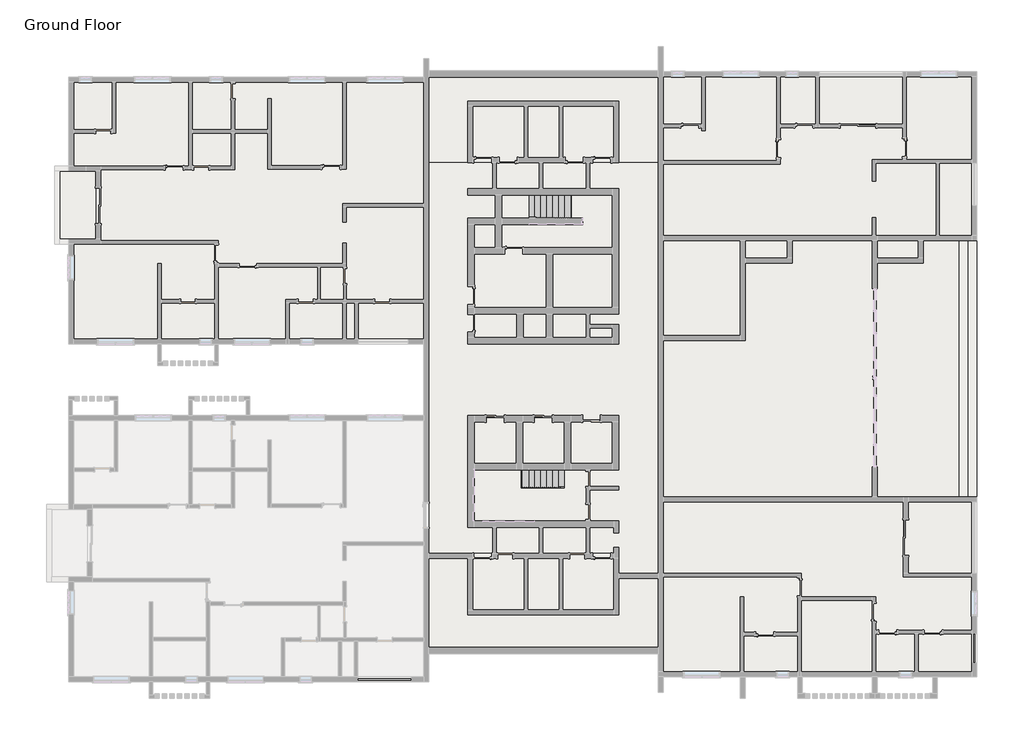
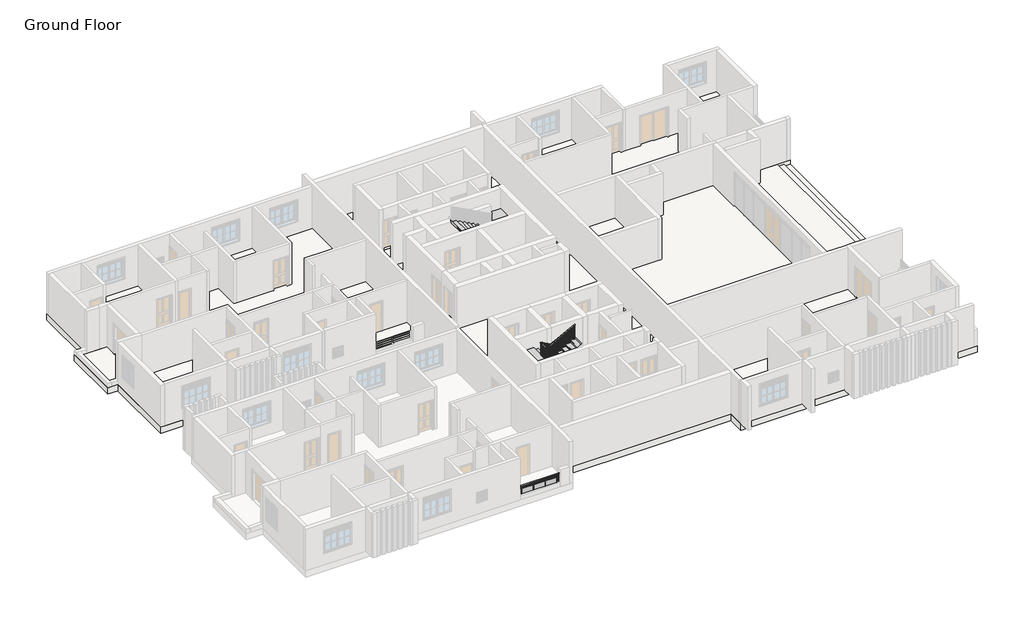
# One storey, part 6 of 9: 12 slabs, 3 railings, 2 stair flights.
"""IFC4 building model written with IfcOpenShell, lengths in millimetres."""

from ifc_helpers import new_model, si_unit, point, frame, frame_2d, origin, origin_with_axes, place, context, project, spatial, polyline, circle_curve, ellipse_curve, trimmed, segment, composite_curve, outline, extrude, faceted_brep, transform, mapped, element, save
from ifc_brep_helpers import plane_surface, extruded_surface, advanced_brep
from components import stair_flight_6b31ae14, stair_flight_54cbe99c

model = new_model("IFC4")

# Units and contexts
model_context = context("Model", 3, world=origin())
ifc_project = project(units=[si_unit("LENGTHUNIT", "METRE", prefix="MILLI")], contexts=[model_context])

# Site, building, storey
site = spatial("IfcSite", under=ifc_project)
building = spatial("IfcBuilding", under=site)
storey = spatial("IfcBuildingStorey", under=building, Name="Ground Floor", Elevation=0.0)

# Railings
placement = place(None, origin())
element("IfcRailing", 1, ObjectType="Glass Panel - Bottom Fill", at=placement, inside=storey, context=model_context, shape_type="SolidModel", body=[
    advanced_brep(
    [(403.2546318, -1832.865108, 914.4), (403.2546318, -1909.065108, 914.4), (3146.4546318, -1832.865108, 914.4), (3146.4546318, -1909.065108, 914.4)],
    [
        (0, 1, ellipse_curve(frame((403.2546318, -1870.965108, 914.4), z_axis=(-1.0, 0.0, 0.0), x_axis=(0.0, -1.0, 0.0)), 38.1, 28.575)),
        (1, 0, ellipse_curve(frame((403.2546318, -1870.965108, 914.4), z_axis=(-1.0, 0.0, 0.0), x_axis=(0.0, -1.0, 0.0)), 38.1, 28.575)),
        (2, 3, ellipse_curve(frame((3146.4546318, -1870.965108, 914.4), z_axis=(1.0, 0.0, 0.0), x_axis=(0.0, -1.0, 0.0)), 38.1, 28.575)),
        (3, 2, ellipse_curve(frame((3146.4546318, -1870.965108, 914.4), z_axis=(1.0, 0.0, 0.0), x_axis=(0.0, -1.0, 0.0)), 38.1, 28.575)),
        (0, 2),
        (3, 1),
    ],
    [
        plane_surface(frame((403.2546318, -1870.965108, 914.4), z_axis=(-1.0, 0.0, 0.0), x_axis=(0.0, 1.0, 0.0))),
        plane_surface(frame((3146.4546318, -1870.965108, 914.4), z_axis=(1.0, 0.0, 0.0), x_axis=(0.0, 1.0, 0.0))),
        extruded_surface(trimmed(ellipse_curve(frame((3146.4546318, -1870.965108, 914.4), z_axis=(-1.0, 0.0, 0.0), x_axis=(0.0, -1.0, 0.0)), 38.1, 28.575), [point((3146.4546318, -1832.865108, 914.4))], [point((3146.4546318, -1909.065108, 914.4))], True, "CARTESIAN"), (-2743.2, 0.0, 0.0), 2743.2),
        extruded_surface(trimmed(ellipse_curve(frame((3146.4546318, -1870.965108, 914.4), z_axis=(-1.0, 0.0, 0.0), x_axis=(0.0, -1.0, 0.0)), 38.1, 28.575), [point((3146.4546318, -1909.065108, 914.4))], [point((3146.4546318, -1832.865108, 914.4))], True, "CARTESIAN"), (-2743.2, 0.0, 0.0), 2743.2),
    ],
    [
        (0, [[1, 2]]),
        (1, [[3, 4]]),
        (2, [[-1, 5, -4, 6]]),
        (3, [[-2, -6, -3, -5]]),
    ],
),
    extrude(outline(polyline([(403.2546318, -1883.665108), (403.2546318, -1858.265108), (3146.4546318, -1858.265108), (3146.4546318, -1883.665108), (403.2546318, -1883.665108)])), frame((0.0, 0.0, 800.1), z_axis=(0.0, 0.0, 1.0), x_axis=(1.0, 0.0, 0.0)), (0.0, 0.0, 1.0), 25.4),
    extrude(outline(polyline([(403.2546318, -1883.665108), (403.2546318, -1858.265108), (3146.4546318, -1858.265108), (3146.4546318, -1883.665108), (403.2546318, -1883.665108)])), frame((0.0, 0.0, 698.5), z_axis=(0.0, 0.0, 1.0), x_axis=(1.0, 0.0, 0.0)), (0.0, 0.0, 1.0), 25.4),
    extrude(outline(polyline([(2987.7046318, -1896.365108), (2987.7046318, -1845.565108), (3000.4046318, -1845.565108), (3000.4046318, -1896.365108), (2987.7046318, -1896.365108)])), origin_with_axes(), (0.0, 0.0, 1.0), 885.825),
    extrude(outline(polyline([(2181.2546318, -1864.429951), (2994.0546318, -1864.429951), (2994.0546318, -1870.779951), (2181.2546318, -1870.779951), (2181.2546318, -1864.429951)])), frame((0.0, 0.0, 101.6), z_axis=(0.0, 0.0, 1.0), x_axis=(1.0, 0.0, 0.0)), (0.0, 0.0, 1.0), 596.9),
    extrude(outline(polyline([(2174.9046318, -1896.365108), (2174.9046318, -1845.565108), (2187.6046318, -1845.565108), (2187.6046318, -1896.365108), (2174.9046318, -1896.365108)])), origin_with_axes(), (0.0, 0.0, 1.0), 885.825),
    extrude(outline(polyline([(1368.4546318, -1864.429951), (2181.2546318, -1864.429951), (2181.2546318, -1870.779951), (1368.4546318, -1870.779951), (1368.4546318, -1864.429951)])), frame((0.0, 0.0, 101.6), z_axis=(0.0, 0.0, 1.0), x_axis=(1.0, 0.0, 0.0)), (0.0, 0.0, 1.0), 596.9),
    extrude(outline(polyline([(1362.1046318, -1896.365108), (1362.1046318, -1845.565108), (1374.8046318, -1845.565108), (1374.8046318, -1896.365108), (1362.1046318, -1896.365108)])), origin_with_axes(), (0.0, 0.0, 1.0), 885.825),
    extrude(outline(polyline([(555.6546318, -1864.429951), (1368.4546318, -1864.429951), (1368.4546318, -1870.779951), (555.6546318, -1870.779951), (555.6546318, -1864.429951)])), frame((0.0, 0.0, 101.6), z_axis=(0.0, 0.0, 1.0), x_axis=(1.0, 0.0, 0.0)), (0.0, 0.0, 1.0), 596.9),
    extrude(outline(polyline([(549.3046318, -1896.365108), (549.3046318, -1845.565108), (562.0046318, -1845.565108), (562.0046318, -1896.365108), (549.3046318, -1896.365108)])), origin_with_axes(), (0.0, 0.0, 1.0), 885.825),
    extrude(outline(polyline([(3133.7546318, -1880.490108), (3133.7546318, -1861.440108), (3152.8046318, -1861.440108), (3152.8046318, -1880.490108), (3133.7546318, -1880.490108)])), origin_with_axes(), (0.0, 0.0, 1.0), 885.825),
    extrude(outline(polyline([(396.9046318, -1880.490108), (396.9046318, -1861.440108), (415.9546318, -1861.440108), (415.9546318, -1880.490108), (396.9046318, -1880.490108)])), origin_with_axes(), (0.0, 0.0, 1.0), 885.825),
])
element("IfcRailing", 2, ObjectType="Handrail - Pipe", at=placement, inside=storey, context=model_context, shape_type="SweptSolid", body=[
    extrude(outline(composite_curve([segment(trimmed(circle_curve(frame_2d((895.35, 31950.0546318)), 19.05), [point((895.35, 31931.0046318))], [point((895.35, 31969.1046318))], False, "CARTESIAN"), True, "CONTINUOUS"), segment(trimmed(circle_curve(frame_2d((895.35, 31950.0546318)), 19.05), [point((895.35, 31969.1046318))], [point((895.35, 31931.0046318))], False, "CARTESIAN"), True, "CONTINUOUS")], self_intersect=False)), frame((0.0, -1007.365108, 0.0), z_axis=(0.0, 1.0, 0.0), x_axis=(0.0, 0.0, 1.0)), (0.0, 0.0, 1.0), 1473.2),
    extrude(outline(composite_curve([segment(trimmed(circle_curve(frame_2d((749.3, 31950.0546318)), 12.7), [point((749.3, 31962.7546318))], [point((749.3, 31937.3546318))], False, "CARTESIAN"), True, "CONTINUOUS"), segment(trimmed(circle_curve(frame_2d((749.3, 31950.0546318)), 12.7), [point((749.3, 31937.3546318))], [point((749.3, 31962.7546318))], False, "CARTESIAN"), True, "CONTINUOUS")], self_intersect=False)), frame((0.0, -1007.365108, 0.0), z_axis=(0.0, 1.0, 0.0), x_axis=(0.0, 0.0, 1.0)), (0.0, 0.0, 1.0), 1473.2),
    extrude(outline(composite_curve([segment(trimmed(circle_curve(frame_2d((596.9, 31950.0546318)), 12.7), [point((596.9, 31962.7546318))], [point((596.9, 31937.3546318))], False, "CARTESIAN"), True, "CONTINUOUS"), segment(trimmed(circle_curve(frame_2d((596.9, 31950.0546318)), 12.7), [point((596.9, 31937.3546318))], [point((596.9, 31962.7546318))], False, "CARTESIAN"), True, "CONTINUOUS")], self_intersect=False)), frame((0.0, -1007.365108, 0.0), z_axis=(0.0, 1.0, 0.0), x_axis=(0.0, 0.0, 1.0)), (0.0, 0.0, 1.0), 1473.2),
    extrude(outline(composite_curve([segment(trimmed(circle_curve(frame_2d((444.5, 31950.0546318)), 12.7), [point((444.5, 31962.7546318))], [point((444.5, 31937.3546318))], False, "CARTESIAN"), True, "CONTINUOUS"), segment(trimmed(circle_curve(frame_2d((444.5, 31950.0546318)), 12.7), [point((444.5, 31937.3546318))], [point((444.5, 31962.7546318))], False, "CARTESIAN"), True, "CONTINUOUS")], self_intersect=False)), frame((0.0, -1007.365108, 0.0), z_axis=(0.0, 1.0, 0.0), x_axis=(0.0, 0.0, 1.0)), (0.0, 0.0, 1.0), 1473.2),
    extrude(outline(composite_curve([segment(trimmed(circle_curve(frame_2d((292.1, 31950.0546318)), 12.7), [point((292.1, 31962.7546318))], [point((292.1, 31937.3546318))], False, "CARTESIAN"), True, "CONTINUOUS"), segment(trimmed(circle_curve(frame_2d((292.1, 31950.0546318)), 12.7), [point((292.1, 31937.3546318))], [point((292.1, 31962.7546318))], False, "CARTESIAN"), True, "CONTINUOUS")], self_intersect=False)), frame((0.0, -1007.365108, 0.0), z_axis=(0.0, 1.0, 0.0), x_axis=(0.0, 0.0, 1.0)), (0.0, 0.0, 1.0), 1473.2),
    extrude(outline(composite_curve([segment(trimmed(circle_curve(frame_2d((139.7, 31950.0546318)), 12.7), [point((139.7, 31962.7546318))], [point((139.7, 31937.3546318))], False, "CARTESIAN"), True, "CONTINUOUS"), segment(trimmed(circle_curve(frame_2d((139.7, 31950.0546318)), 12.7), [point((139.7, 31937.3546318))], [point((139.7, 31962.7546318))], False, "CARTESIAN"), True, "CONTINUOUS")], self_intersect=False)), frame((0.0, -1007.365108, 0.0), z_axis=(0.0, 1.0, 0.0), x_axis=(0.0, 0.0, 1.0)), (0.0, 0.0, 1.0), 1473.2),
    extrude(outline(composite_curve([segment(trimmed(circle_curve(frame_2d((31950.0546318, -753.365108)), 12.7), [point((31962.7546318, -753.365108))], [point((31937.3546318, -753.365108))], False, "CARTESIAN"), True, "CONTINUOUS"), segment(trimmed(circle_curve(frame_2d((31950.0546318, -753.365108)), 12.7), [point((31937.3546318, -753.365108))], [point((31962.7546318, -753.365108))], False, "CARTESIAN"), True, "CONTINUOUS")], self_intersect=False)), origin_with_axes(), (0.0, 0.0, 1.0), 876.3),
    extrude(outline(composite_curve([segment(trimmed(circle_curve(frame_2d((31950.0546318, -994.665108)), 12.7), [point((31962.7546318, -994.665108))], [point((31937.3546318, -994.665108))], False, "CARTESIAN"), True, "CONTINUOUS"), segment(trimmed(circle_curve(frame_2d((31950.0546318, -994.665108)), 12.7), [point((31937.3546318, -994.665108))], [point((31962.7546318, -994.665108))], False, "CARTESIAN"), True, "CONTINUOUS")], self_intersect=False)), origin_with_axes(), (0.0, 0.0, 1.0), 876.3),
    extrude(outline(composite_curve([segment(trimmed(circle_curve(frame_2d((31950.0546318, 453.134892)), 12.7), [point((31962.7546318, 453.134892))], [point((31937.3546318, 453.134892))], False, "CARTESIAN"), True, "CONTINUOUS"), segment(trimmed(circle_curve(frame_2d((31950.0546318, 453.134892)), 12.7), [point((31937.3546318, 453.134892))], [point((31962.7546318, 453.134892))], False, "CARTESIAN"), True, "CONTINUOUS")], self_intersect=False)), origin_with_axes(), (0.0, 0.0, 1.0), 876.3),
])
element("IfcRailing", 3, ObjectType="Handrail - Rectangular", at=placement, inside=storey, context=model_context, shape_type="SolidModel", body=[
    faceted_brep([(10969.6546318, 7933.434892, 1082.8421053), (10969.6546318, 7933.434892, 1024.9027862), (10969.6546318, 7984.234892, 1024.9027862), (10969.6546318, 7984.234892, 1082.8421053), (7667.6546318, 7933.434892, 2893.9113573), (7616.8546318, 7933.434892, 2863.8346421), (7616.8546318, 7984.234892, 2863.8346421), (7667.6546318, 7984.234892, 2893.9113573), (7667.6546318, 7933.434892, 2935.7052632), (7616.8546318, 7933.434892, 2884.9052632), (7616.8546318, 7984.234892, 2884.9052632), (7667.6546318, 7984.234892, 2935.7052632), (7591.4546318, 7933.434892, 2935.7052632), (7591.4546318, 7933.434892, 2884.9052632), (7540.6546318, 7984.234892, 2884.9052632), (7540.6546318, 7984.234892, 2935.7052632), (7591.4546318, 7857.234892, 2935.7052632), (7591.4546318, 7857.234892, 2884.9052632), (7540.6546318, 7857.234892, 2884.9052632), (7540.6546318, 7857.234892, 2935.7052632), (7591.4546318, 7247.634892, 2935.7052632), (7591.4546318, 7196.834892, 2884.9052632), (7540.6546318, 7196.834892, 2884.9052632), (7540.6546318, 7247.634892, 2935.7052632), (7591.4546318, 7247.634892, 3145.6810382), (7591.4546318, 7196.834892, 3094.8810382), (7540.6546318, 7196.834892, 3094.8810382), (7540.6546318, 7247.634892, 3145.6810382), (7591.4546318, 7171.434892, 3145.6810382), (7591.4546318, 7171.434892, 3094.8810382), (7540.6546318, 7120.634892, 3094.8810382), (7540.6546318, 7120.634892, 3145.6810382), (7667.6546318, 7171.434892, 3145.6810382), (7680.6001277, 7171.434892, 3094.8810382), (7680.6001277, 7120.634892, 3094.8810382), (7667.6546318, 7120.634892, 3145.6810382), (9445.6546318, 7171.434892, 4114.8), (9445.6546318, 7120.634892, 4114.8), (9445.6546318, 7120.634892, 4056.9439114), (9445.6546318, 7171.434892, 4056.9439114)], [[[0, 1, 2, 3]], [[1, 0, 4, 5]], [[2, 1, 5, 6]], [[3, 2, 6, 7]], [[0, 3, 7, 4]], [[5, 4, 8, 9]], [[6, 5, 9, 10]], [[7, 6, 10, 11]], [[4, 7, 11, 8]], [[9, 8, 12, 13]], [[10, 9, 13, 14]], [[11, 10, 14, 15]], [[8, 11, 15, 12]], [[13, 12, 16, 17]], [[14, 13, 17, 18]], [[15, 14, 18, 19]], [[12, 15, 19, 16]], [[17, 16, 20, 21]], [[18, 17, 21, 22]], [[19, 18, 22, 23]], [[16, 19, 23, 20]], [[21, 20, 24, 25]], [[22, 21, 25, 26]], [[23, 22, 26, 27]], [[20, 23, 27, 24]], [[25, 24, 28, 29]], [[26, 25, 29, 30]], [[27, 26, 30, 31]], [[24, 27, 31, 28]], [[29, 28, 32, 33]], [[30, 29, 33, 34]], [[31, 30, 34, 35]], [[28, 31, 35, 32]], [[36, 37, 38, 39]], [[33, 32, 36, 39]], [[34, 33, 39, 38]], [[35, 34, 38, 37]], [[32, 35, 37, 36]]]),
    extrude(outline(polyline([(4024.0630895, 9385.3296318), (3031.9578947, 9385.3296318), (3031.9578947, 9404.3796318), (4034.4465069, 9404.3796318), (4024.0630895, 9385.3296318)])), frame((0.0, 7136.509892, 0.0), z_axis=(0.0, 1.0, 0.0), x_axis=(0.0, 0.0, 1.0)), (0.0, 0.0, 1.0), 19.05),
    extrude(outline(polyline([(3968.6848631, 9283.7296318), (3031.9578947, 9283.7296318), (3031.9578947, 9302.7796318), (3979.0682805, 9302.7796318), (3968.6848631, 9283.7296318)])), frame((0.0, 7136.509892, 0.0), z_axis=(0.0, 1.0, 0.0), x_axis=(0.0, 0.0, 1.0)), (0.0, 0.0, 1.0), 19.05),
    extrude(outline(polyline([(3913.3066367, 9182.1296318), (3031.9578947, 9182.1296318), (3031.9578947, 9201.1796318), (3923.6900541, 9201.1796318), (3913.3066367, 9182.1296318)])), frame((0.0, 7136.509892, 0.0), z_axis=(0.0, 1.0, 0.0), x_axis=(0.0, 0.0, 1.0)), (0.0, 0.0, 1.0), 19.05),
    extrude(outline(polyline([(3857.9284103, 9080.5296318), (2863.5157895, 9080.5296318), (2863.5157895, 9099.5796318), (3868.3118278, 9099.5796318), (3857.9284103, 9080.5296318)])), frame((0.0, 7136.509892, 0.0), z_axis=(0.0, 1.0, 0.0), x_axis=(0.0, 0.0, 1.0)), (0.0, 0.0, 1.0), 19.05),
    extrude(outline(polyline([(3802.5501839, 8978.9296318), (2863.5157895, 8978.9296318), (2863.5157895, 8997.9796318), (3812.9336014, 8997.9796318), (3802.5501839, 8978.9296318)])), frame((0.0, 7136.509892, 0.0), z_axis=(0.0, 1.0, 0.0), x_axis=(0.0, 0.0, 1.0)), (0.0, 0.0, 1.0), 19.05),
    extrude(outline(polyline([(3747.1719575, 8877.3296318), (2863.5157895, 8877.3296318), (2863.5157895, 8896.3796318), (3757.555375, 8896.3796318), (3747.1719575, 8877.3296318)])), frame((0.0, 7136.509892, 0.0), z_axis=(0.0, 1.0, 0.0), x_axis=(0.0, 0.0, 1.0)), (0.0, 0.0, 1.0), 19.05),
    extrude(outline(polyline([(3691.7937311, 8775.7296318), (2695.0736842, 8775.7296318), (2695.0736842, 8794.7796318), (3702.1771486, 8794.7796318), (3691.7937311, 8775.7296318)])), frame((0.0, 7136.509892, 0.0), z_axis=(0.0, 1.0, 0.0), x_axis=(0.0, 0.0, 1.0)), (0.0, 0.0, 1.0), 19.05),
    extrude(outline(polyline([(3636.4155048, 8674.1296318), (2695.0736842, 8674.1296318), (2695.0736842, 8693.1796318), (3646.7989222, 8693.1796318), (3636.4155048, 8674.1296318)])), frame((0.0, 7136.509892, 0.0), z_axis=(0.0, 1.0, 0.0), x_axis=(0.0, 0.0, 1.0)), (0.0, 0.0, 1.0), 19.05),
    extrude(outline(polyline([(3581.0372784, 8572.5296318), (2695.0736842, 8572.5296318), (2695.0736842, 8591.5796318), (3591.4206958, 8591.5796318), (3581.0372784, 8572.5296318)])), frame((0.0, 7136.509892, 0.0), z_axis=(0.0, 1.0, 0.0), x_axis=(0.0, 0.0, 1.0)), (0.0, 0.0, 1.0), 19.05),
    extrude(outline(polyline([(3525.659052, 8470.9296318), (2526.6315789, 8470.9296318), (2526.6315789, 8489.9796318), (3536.0424694, 8489.9796318), (3525.659052, 8470.9296318)])), frame((0.0, 7136.509892, 0.0), z_axis=(0.0, 1.0, 0.0), x_axis=(0.0, 0.0, 1.0)), (0.0, 0.0, 1.0), 19.05),
    extrude(outline(polyline([(3470.2808256, 8369.3296318), (2526.6315789, 8369.3296318), (2526.6315789, 8388.3796318), (3480.664243, 8388.3796318), (3470.2808256, 8369.3296318)])), frame((0.0, 7136.509892, 0.0), z_axis=(0.0, 1.0, 0.0), x_axis=(0.0, 0.0, 1.0)), (0.0, 0.0, 1.0), 19.05),
    extrude(outline(polyline([(3414.9025992, 8267.7296318), (2526.6315789, 8267.7296318), (2526.6315789, 8286.7796318), (3425.2860167, 8286.7796318), (3414.9025992, 8267.7296318)])), frame((0.0, 7136.509892, 0.0), z_axis=(0.0, 1.0, 0.0), x_axis=(0.0, 0.0, 1.0)), (0.0, 0.0, 1.0), 19.05),
    extrude(outline(polyline([(3359.5243728, 8166.1296318), (2358.1894737, 8166.1296318), (2358.1894737, 8185.1796318), (3369.9077903, 8185.1796318), (3359.5243728, 8166.1296318)])), frame((0.0, 7136.509892, 0.0), z_axis=(0.0, 1.0, 0.0), x_axis=(0.0, 0.0, 1.0)), (0.0, 0.0, 1.0), 19.05),
    extrude(outline(polyline([(3304.1461464, 8064.5296318), (2358.1894737, 8064.5296318), (2358.1894737, 8083.5796318), (3314.5295639, 8083.5796318), (3304.1461464, 8064.5296318)])), frame((0.0, 7136.509892, 0.0), z_axis=(0.0, 1.0, 0.0), x_axis=(0.0, 0.0, 1.0)), (0.0, 0.0, 1.0), 19.05),
    extrude(outline(polyline([(3248.76792, 7962.9296318), (2358.1894737, 7962.9296318), (2358.1894737, 7981.9796318), (3259.1513375, 7981.9796318), (3248.76792, 7962.9296318)])), frame((0.0, 7136.509892, 0.0), z_axis=(0.0, 1.0, 0.0), x_axis=(0.0, 0.0, 1.0)), (0.0, 0.0, 1.0), 19.05),
    extrude(outline(polyline([(3193.3896937, 7861.3296318), (2189.7473684, 7861.3296318), (2189.7473684, 7880.3796318), (3203.7731111, 7880.3796318), (3193.3896937, 7861.3296318)])), frame((0.0, 7136.509892, 0.0), z_axis=(0.0, 1.0, 0.0), x_axis=(0.0, 0.0, 1.0)), (0.0, 0.0, 1.0), 19.05),
    extrude(outline(polyline([(3138.0114673, 7759.7296318), (2189.7473684, 7759.7296318), (2189.7473684, 7778.7796318), (3148.3948847, 7778.7796318), (3138.0114673, 7759.7296318)])), frame((0.0, 7136.509892, 0.0), z_axis=(0.0, 1.0, 0.0), x_axis=(0.0, 0.0, 1.0)), (0.0, 0.0, 1.0), 19.05),
    extrude(outline(polyline([(3082.6332409, 7658.1296318), (2189.7473684, 7658.1296318), (2189.7473684, 7677.1796318), (3093.0166583, 7677.1796318), (3082.6332409, 7658.1296318)])), frame((0.0, 7136.509892, 0.0), z_axis=(0.0, 1.0, 0.0), x_axis=(0.0, 0.0, 1.0)), (0.0, 0.0, 1.0), 19.05),
    extrude(outline(polyline([(7575.5796318, 7257.159892), (7575.5796318, 7238.109892), (7556.5296318, 7238.109892), (7556.5296318, 7257.159892), (7575.5796318, 7257.159892)])), frame((0.0, 0.0, 2021.3052632), z_axis=(0.0, 0.0, 1.0), x_axis=(1.0, 0.0, 0.0)), (0.0, 0.0, 1.0), 863.6),
    extrude(outline(polyline([(7575.5796318, 7358.759892), (7575.5796318, 7339.709892), (7556.5296318, 7339.709892), (7556.5296318, 7358.759892), (7575.5796318, 7358.759892)])), frame((0.0, 0.0, 2021.3052632), z_axis=(0.0, 0.0, 1.0), x_axis=(1.0, 0.0, 0.0)), (0.0, 0.0, 1.0), 863.6),
    extrude(outline(polyline([(7575.5796318, 7460.359892), (7575.5796318, 7441.309892), (7556.5296318, 7441.309892), (7556.5296318, 7460.359892), (7575.5796318, 7460.359892)])), frame((0.0, 0.0, 2021.3052632), z_axis=(0.0, 0.0, 1.0), x_axis=(1.0, 0.0, 0.0)), (0.0, 0.0, 1.0), 863.6),
    extrude(outline(polyline([(7575.5796318, 7561.959892), (7575.5796318, 7542.909892), (7556.5296318, 7542.909892), (7556.5296318, 7561.959892), (7575.5796318, 7561.959892)])), frame((0.0, 0.0, 2021.3052632), z_axis=(0.0, 0.0, 1.0), x_axis=(1.0, 0.0, 0.0)), (0.0, 0.0, 1.0), 863.6),
    extrude(outline(polyline([(7575.5796318, 7663.559892), (7575.5796318, 7644.509892), (7556.5296318, 7644.509892), (7556.5296318, 7663.559892), (7575.5796318, 7663.559892)])), frame((0.0, 0.0, 2021.3052632), z_axis=(0.0, 0.0, 1.0), x_axis=(1.0, 0.0, 0.0)), (0.0, 0.0, 1.0), 863.6),
    extrude(outline(polyline([(7575.5796318, 7765.159892), (7575.5796318, 7746.109892), (7556.5296318, 7746.109892), (7556.5296318, 7765.159892), (7575.5796318, 7765.159892)])), frame((0.0, 0.0, 2021.3052632), z_axis=(0.0, 0.0, 1.0), x_axis=(1.0, 0.0, 0.0)), (0.0, 0.0, 1.0), 863.6),
    extrude(outline(polyline([(7575.5796318, 7866.759892), (7575.5796318, 7847.709892), (7556.5296318, 7847.709892), (7556.5296318, 7866.759892), (7575.5796318, 7866.759892)])), frame((0.0, 0.0, 2021.3052632), z_axis=(0.0, 0.0, 1.0), x_axis=(1.0, 0.0, 0.0)), (0.0, 0.0, 1.0), 863.6),
    extrude(outline(polyline([(7626.3796318, 7949.309892), (7607.3296318, 7949.309892), (7607.3296318, 7968.359892), (7626.3796318, 7968.359892), (7626.3796318, 7949.309892)])), frame((0.0, 0.0, 1852.8631579), z_axis=(0.0, 0.0, 1.0), x_axis=(1.0, 0.0, 0.0)), (0.0, 0.0, 1.0), 1032.0421053),
    extrude(outline(polyline([(2813.3336726, 7708.9296318), (1852.8631579, 7708.9296318), (1852.8631579, 7727.9796318), (2802.8851962, 7727.9796318), (2813.3336726, 7708.9296318)])), frame((0.0, 7949.309892, 0.0), z_axis=(0.0, 1.0, 0.0), x_axis=(0.0, 0.0, 1.0)), (0.0, 0.0, 1.0), 19.05),
    extrude(outline(polyline([(2757.6084649, 7810.5296318), (1852.8631579, 7810.5296318), (1852.8631579, 7829.5796318), (2747.1599884, 7829.5796318), (2757.6084649, 7810.5296318)])), frame((0.0, 7949.309892, 0.0), z_axis=(0.0, 1.0, 0.0), x_axis=(0.0, 0.0, 1.0)), (0.0, 0.0, 1.0), 19.05),
    extrude(outline(polyline([(2701.8832571, 7912.1296318), (1684.4210526, 7912.1296318), (1684.4210526, 7931.1796318), (2691.4347806, 7931.1796318), (2701.8832571, 7912.1296318)])), frame((0.0, 7949.309892, 0.0), z_axis=(0.0, 1.0, 0.0), x_axis=(0.0, 0.0, 1.0)), (0.0, 0.0, 1.0), 19.05),
    extrude(outline(polyline([(2646.1580493, 8013.7296318), (1684.4210526, 8013.7296318), (1684.4210526, 8032.7796318), (2635.7095729, 8032.7796318), (2646.1580493, 8013.7296318)])), frame((0.0, 7949.309892, 0.0), z_axis=(0.0, 1.0, 0.0), x_axis=(0.0, 0.0, 1.0)), (0.0, 0.0, 1.0), 19.05),
    extrude(outline(polyline([(2590.4328416, 8115.3296318), (1684.4210526, 8115.3296318), (1684.4210526, 8134.3796318), (2579.9843651, 8134.3796318), (2590.4328416, 8115.3296318)])), frame((0.0, 7949.309892, 0.0), z_axis=(0.0, 1.0, 0.0), x_axis=(0.0, 0.0, 1.0)), (0.0, 0.0, 1.0), 19.05),
    extrude(outline(polyline([(2534.7076338, 8216.9296318), (1515.9789474, 8216.9296318), (1515.9789474, 8235.9796318), (2524.2591574, 8235.9796318), (2534.7076338, 8216.9296318)])), frame((0.0, 7949.309892, 0.0), z_axis=(0.0, 1.0, 0.0), x_axis=(0.0, 0.0, 1.0)), (0.0, 0.0, 1.0), 19.05),
    extrude(outline(polyline([(2478.9824261, 8318.5296318), (1515.9789474, 8318.5296318), (1515.9789474, 8337.5796318), (2468.5339496, 8337.5796318), (2478.9824261, 8318.5296318)])), frame((0.0, 7949.309892, 0.0), z_axis=(0.0, 1.0, 0.0), x_axis=(0.0, 0.0, 1.0)), (0.0, 0.0, 1.0), 19.05),
    extrude(outline(polyline([(2423.2572183, 8420.1296318), (1515.9789474, 8420.1296318), (1515.9789474, 8439.1796318), (2412.8087419, 8439.1796318), (2423.2572183, 8420.1296318)])), frame((0.0, 7949.309892, 0.0), z_axis=(0.0, 1.0, 0.0), x_axis=(0.0, 0.0, 1.0)), (0.0, 0.0, 1.0), 19.05),
    extrude(outline(polyline([(2367.5320106, 8521.7296318), (1347.5368421, 8521.7296318), (1347.5368421, 8540.7796318), (2357.0835341, 8540.7796318), (2367.5320106, 8521.7296318)])), frame((0.0, 7949.309892, 0.0), z_axis=(0.0, 1.0, 0.0), x_axis=(0.0, 0.0, 1.0)), (0.0, 0.0, 1.0), 19.05),
    extrude(outline(polyline([(2311.8068028, 8623.3296318), (1347.5368421, 8623.3296318), (1347.5368421, 8642.3796318), (2301.3583264, 8642.3796318), (2311.8068028, 8623.3296318)])), frame((0.0, 7949.309892, 0.0), z_axis=(0.0, 1.0, 0.0), x_axis=(0.0, 0.0, 1.0)), (0.0, 0.0, 1.0), 19.05),
    extrude(outline(polyline([(2256.0815951, 8724.9296318), (1347.5368421, 8724.9296318), (1347.5368421, 8743.9796318), (2245.6331186, 8743.9796318), (2256.0815951, 8724.9296318)])), frame((0.0, 7949.309892, 0.0), z_axis=(0.0, 1.0, 0.0), x_axis=(0.0, 0.0, 1.0)), (0.0, 0.0, 1.0), 19.05),
    extrude(outline(polyline([(2200.3563873, 8826.5296318), (1179.0947368, 8826.5296318), (1179.0947368, 8845.5796318), (2189.9079108, 8845.5796318), (2200.3563873, 8826.5296318)])), frame((0.0, 7949.309892, 0.0), z_axis=(0.0, 1.0, 0.0), x_axis=(0.0, 0.0, 1.0)), (0.0, 0.0, 1.0), 19.05),
    extrude(outline(polyline([(2144.6311795, 8928.1296318), (1179.0947368, 8928.1296318), (1179.0947368, 8947.1796318), (2134.1827031, 8947.1796318), (2144.6311795, 8928.1296318)])), frame((0.0, 7949.309892, 0.0), z_axis=(0.0, 1.0, 0.0), x_axis=(0.0, 0.0, 1.0)), (0.0, 0.0, 1.0), 19.05),
    extrude(outline(polyline([(2088.9059718, 9029.7296318), (1179.0947368, 9029.7296318), (1179.0947368, 9048.7796318), (2078.4574953, 9048.7796318), (2088.9059718, 9029.7296318)])), frame((0.0, 7949.309892, 0.0), z_axis=(0.0, 1.0, 0.0), x_axis=(0.0, 0.0, 1.0)), (0.0, 0.0, 1.0), 19.05),
    extrude(outline(polyline([(2033.180764, 9131.3296318), (1179.0947368, 9131.3296318), (1179.0947368, 9150.3796318), (2022.7322876, 9150.3796318), (2033.180764, 9131.3296318)])), frame((0.0, 7949.309892, 0.0), z_axis=(0.0, 1.0, 0.0), x_axis=(0.0, 0.0, 1.0)), (0.0, 0.0, 1.0), 19.05),
    extrude(outline(polyline([(1977.4555563, 9232.9296318), (1010.6526316, 9232.9296318), (1010.6526316, 9251.9796318), (1967.0070798, 9251.9796318), (1977.4555563, 9232.9296318)])), frame((0.0, 7949.309892, 0.0), z_axis=(0.0, 1.0, 0.0), x_axis=(0.0, 0.0, 1.0)), (0.0, 0.0, 1.0), 19.05),
    extrude(outline(polyline([(1921.7303485, 9334.5296318), (1010.6526316, 9334.5296318), (1010.6526316, 9353.5796318), (1911.2818721, 9353.5796318), (1921.7303485, 9334.5296318)])), frame((0.0, 7949.309892, 0.0), z_axis=(0.0, 1.0, 0.0), x_axis=(0.0, 0.0, 1.0)), (0.0, 0.0, 1.0), 19.05),
    extrude(outline(polyline([(1866.0051408, 9436.1296318), (1010.6526316, 9436.1296318), (1010.6526316, 9455.1796318), (1855.5566643, 9455.1796318), (1866.0051408, 9436.1296318)])), frame((0.0, 7949.309892, 0.0), z_axis=(0.0, 1.0, 0.0), x_axis=(0.0, 0.0, 1.0)), (0.0, 0.0, 1.0), 19.05),
    extrude(outline(polyline([(1810.279933, 9537.7296318), (842.2105263, 9537.7296318), (842.2105263, 9556.7796318), (1799.8314565, 9556.7796318), (1810.279933, 9537.7296318)])), frame((0.0, 7949.309892, 0.0), z_axis=(0.0, 1.0, 0.0), x_axis=(0.0, 0.0, 1.0)), (0.0, 0.0, 1.0), 19.05),
    extrude(outline(polyline([(1754.5547252, 9639.3296318), (842.2105263, 9639.3296318), (842.2105263, 9658.3796318), (1744.1062488, 9658.3796318), (1754.5547252, 9639.3296318)])), frame((0.0, 7949.309892, 0.0), z_axis=(0.0, 1.0, 0.0), x_axis=(0.0, 0.0, 1.0)), (0.0, 0.0, 1.0), 19.05),
    extrude(outline(polyline([(1698.8295175, 9740.9296318), (842.2105263, 9740.9296318), (842.2105263, 9759.9796318), (1688.381041, 9759.9796318), (1698.8295175, 9740.9296318)])), frame((0.0, 7949.309892, 0.0), z_axis=(0.0, 1.0, 0.0), x_axis=(0.0, 0.0, 1.0)), (0.0, 0.0, 1.0), 19.05),
    extrude(outline(polyline([(1643.1043097, 9842.5296318), (673.7684211, 9842.5296318), (673.7684211, 9861.5796318), (1632.6558333, 9861.5796318), (1643.1043097, 9842.5296318)])), frame((0.0, 7949.309892, 0.0), z_axis=(0.0, 1.0, 0.0), x_axis=(0.0, 0.0, 1.0)), (0.0, 0.0, 1.0), 19.05),
    extrude(outline(polyline([(1587.379102, 9944.1296318), (673.7684211, 9944.1296318), (673.7684211, 9963.1796318), (1576.9306255, 9963.1796318), (1587.379102, 9944.1296318)])), frame((0.0, 7949.309892, 0.0), z_axis=(0.0, 1.0, 0.0), x_axis=(0.0, 0.0, 1.0)), (0.0, 0.0, 1.0), 19.05),
    extrude(outline(polyline([(1531.6538942, 10045.7296318), (673.7684211, 10045.7296318), (673.7684211, 10064.7796318), (1521.2054178, 10064.7796318), (1531.6538942, 10045.7296318)])), frame((0.0, 7949.309892, 0.0), z_axis=(0.0, 1.0, 0.0), x_axis=(0.0, 0.0, 1.0)), (0.0, 0.0, 1.0), 19.05),
    extrude(outline(polyline([(1475.9286865, 10147.3296318), (505.3263158, 10147.3296318), (505.3263158, 10166.3796318), (1465.48021, 10166.3796318), (1475.9286865, 10147.3296318)])), frame((0.0, 7949.309892, 0.0), z_axis=(0.0, 1.0, 0.0), x_axis=(0.0, 0.0, 1.0)), (0.0, 0.0, 1.0), 19.05),
    extrude(outline(polyline([(1420.2034787, 10248.9296318), (505.3263158, 10248.9296318), (505.3263158, 10267.9796318), (1409.7550023, 10267.9796318), (1420.2034787, 10248.9296318)])), frame((0.0, 7949.309892, 0.0), z_axis=(0.0, 1.0, 0.0), x_axis=(0.0, 0.0, 1.0)), (0.0, 0.0, 1.0), 19.05),
    extrude(outline(polyline([(1364.478271, 10350.5296318), (505.3263158, 10350.5296318), (505.3263158, 10369.5796318), (1354.0297945, 10369.5796318), (1364.478271, 10350.5296318)])), frame((0.0, 7949.309892, 0.0), z_axis=(0.0, 1.0, 0.0), x_axis=(0.0, 0.0, 1.0)), (0.0, 0.0, 1.0), 19.05),
    extrude(outline(polyline([(1308.7530632, 10452.1296318), (336.8842105, 10452.1296318), (336.8842105, 10471.1796318), (1298.3045867, 10471.1796318), (1308.7530632, 10452.1296318)])), frame((0.0, 7949.309892, 0.0), z_axis=(0.0, 1.0, 0.0), x_axis=(0.0, 0.0, 1.0)), (0.0, 0.0, 1.0), 19.05),
    extrude(outline(polyline([(1253.0278554, 10553.7296318), (336.8842105, 10553.7296318), (336.8842105, 10572.7796318), (1242.579379, 10572.7796318), (1253.0278554, 10553.7296318)])), frame((0.0, 7949.309892, 0.0), z_axis=(0.0, 1.0, 0.0), x_axis=(0.0, 0.0, 1.0)), (0.0, 0.0, 1.0), 19.05),
    extrude(outline(polyline([(1197.3026477, 10655.3296318), (336.8842105, 10655.3296318), (336.8842105, 10674.3796318), (1186.8541712, 10674.3796318), (1197.3026477, 10655.3296318)])), frame((0.0, 7949.309892, 0.0), z_axis=(0.0, 1.0, 0.0), x_axis=(0.0, 0.0, 1.0)), (0.0, 0.0, 1.0), 19.05),
    extrude(outline(polyline([(1141.5774399, 10756.9296318), (168.4421053, 10756.9296318), (168.4421053, 10775.9796318), (1131.1289635, 10775.9796318), (1141.5774399, 10756.9296318)])), frame((0.0, 7949.309892, 0.0), z_axis=(0.0, 1.0, 0.0), x_axis=(0.0, 0.0, 1.0)), (0.0, 0.0, 1.0), 19.05),
    extrude(outline(polyline([(1085.8522322, 10858.5296318), (168.4421053, 10858.5296318), (168.4421053, 10877.5796318), (1075.4037557, 10877.5796318), (1085.8522322, 10858.5296318)])), frame((0.0, 7949.309892, 0.0), z_axis=(0.0, 1.0, 0.0), x_axis=(0.0, 0.0, 1.0)), (0.0, 0.0, 1.0), 19.05),
    extrude(outline(polyline([(7575.5796318, 7155.559892), (7575.5796318, 7136.509892), (7556.5296318, 7136.509892), (7556.5296318, 7155.559892), (7575.5796318, 7155.559892)])), frame((0.0, 0.0, 2021.3052632), z_axis=(0.0, 0.0, 1.0), x_axis=(1.0, 0.0, 0.0)), (0.0, 0.0, 1.0), 1073.5757751),
    extrude(outline(polyline([(7575.5796318, 7949.309892), (7556.5296318, 7949.309892), (7556.5296318, 7968.359892), (7575.5796318, 7968.359892), (7575.5796318, 7949.309892)])), frame((0.0, 0.0, 2021.3052632), z_axis=(0.0, 0.0, 1.0), x_axis=(1.0, 0.0, 0.0)), (0.0, 0.0, 1.0), 863.6),
    extrude(outline(polyline([(4046.5604939, 9426.6046318), (3031.9578947, 9426.6046318), (3031.9578947, 9445.6546318), (4056.9439114, 9445.6546318), (4046.5604939, 9426.6046318)])), frame((0.0, 7136.509892, 0.0), z_axis=(0.0, 1.0, 0.0), x_axis=(0.0, 0.0, 1.0)), (0.0, 0.0, 1.0), 19.05),
    extrude(outline(polyline([(1035.3512626, 10950.6046318), (168.4421053, 10950.6046318), (168.4421053, 10969.6546318), (1024.9027862, 10969.6546318), (1035.3512626, 10950.6046318)])), frame((0.0, 7949.309892, 0.0), z_axis=(0.0, 1.0, 0.0), x_axis=(0.0, 0.0, 1.0)), (0.0, 0.0, 1.0), 19.05),
])

# Slabs
element("IfcSlab", 4, at=placement, inside=storey, context=model_context, shape_type="Brep", body=[
    faceted_brep([(31619.8546318, 20608.034892, -304.8), (31619.8546318, 7476.234892, -304.8), (16024.2546318, 7476.234892, -304.8), (16024.2546318, 20608.034892, -304.8), (31619.8546318, 20608.034892, -152.4), (31162.6546318, 20608.034892, -152.4), (16024.2546318, 20608.034892, -152.4), (16024.2546318, 7476.234892, -152.4), (31162.6546318, 7476.234892, -152.4), (31619.8546318, 7476.234892, -152.4)], [[[0, 1, 2, 3]], [[4, 5, 6, 7, 8, 9]], [[1, 0, 4, 9]], [[2, 1, 9, 8, 7]], [[3, 2, 7, 6]], [[0, 3, 6, 5, 4]]]),
])
element("IfcSlab", 5, at=placement, inside=storey, context=model_context, shape_type="Brep", body=[
    faceted_brep([(32077.0546318, 20608.034892, -457.2), (32077.0546318, 7476.234892, -457.2), (16024.2546318, 7476.234892, -457.2), (16024.2546318, 20608.034892, -457.2), (32077.0546318, 20608.034892, -304.8), (31619.8546318, 20608.034892, -304.8), (16024.2546318, 20608.034892, -304.8), (16024.2546318, 7476.234892, -304.8), (31619.8546318, 7476.234892, -304.8), (32077.0546318, 7476.234892, -304.8)], [[[0, 1, 2, 3]], [[4, 5, 6, 7, 8, 9]], [[1, 0, 4, 9]], [[2, 1, 9, 8, 7]], [[3, 2, 7, 6]], [[0, 3, 6, 5, 4]]]),
])
element("IfcSlab", 6, ObjectType="18\"", at=placement, inside=storey, context=model_context, shape_type="Brep", body=[
    faceted_brep([(15770.2546318, 24595.834892, -457.2), (15770.2546318, 4580.634892, -457.2), (15770.2546318, 3564.634892, -457.2), (13763.6546318, 3564.634892, -457.2), (13763.6546318, 4580.634892, -457.2), (4035.4546318, 4580.634892, -457.2), (4035.4546318, 24595.834892, -457.2), (15770.2546318, 24595.834892, 0.0), (12265.0546318, 24595.834892, 0.0), (12087.2546318, 24595.834892, 0.0), (9877.4546318, 24595.834892, 0.0), (9699.6546318, 24595.834892, 0.0), (7489.8546318, 24595.834892, 0.0), (7312.0546318, 24595.834892, 0.0), (4035.4546318, 24595.834892, 0.0), (4035.4546318, 4580.634892, 0.0), (7312.0546318, 4580.634892, 0.0), (7489.8546318, 4580.634892, 0.0), (9699.6546318, 4580.634892, 0.0), (9877.4546318, 4580.634892, 0.0), (12087.2546318, 4580.634892, 0.0), (12265.0546318, 4580.634892, 0.0), (13763.6546318, 4580.634892, 0.0), (13763.6546318, 3564.634892, 0.0), (15770.2546318, 3564.634892, 0.0), (15770.2546318, 4580.634892, 0.0)], [[[0, 1, 2, 3, 4, 5, 6]], [[7, 8, 9, 10, 11, 12, 13, 14, 15, 16, 17, 18, 19, 20, 21, 22, 23, 24, 25]], [[1, 0, 7, 25]], [[5, 4, 22, 21, 20, 19, 18, 17, 16, 15]], [[6, 5, 15, 14]], [[0, 6, 14, 13, 12, 11, 10, 9, 8, 7]], [[2, 1, 25, 24]], [[3, 2, 24, 23]], [[4, 3, 23, 22]]]),
])
element("IfcSlab", 7, ObjectType="Deck", at=placement, inside=storey, context=model_context, shape_type="Brep", body=[
    faceted_brep([(-14392.2453682, 24418.034892, -457.2), (-14392.2453682, 24164.034892, -457.2), (-13007.9453682, 24164.034892, -457.2), (-13007.9453682, 20684.234892, -457.2), (-14392.2453682, 20684.234892, -457.2), (-14392.2453682, 20430.234892, -457.2), (-15090.7453682, 20430.234892, -457.2), (-15090.7453682, 24418.034892, -457.2), (-14392.2453682, 24418.034892, 0.0), (-15090.7453682, 24418.034892, 0.0), (-15090.7453682, 24164.034892, 0.0), (-15090.7453682, 20430.234892, 0.0), (-14836.7453682, 20430.234892, 0.0), (-14392.2453682, 20430.234892, 0.0), (-14392.2453682, 20684.234892, 0.0), (-13007.9453682, 20684.234892, 0.0), (-13007.9453682, 24164.034892, 0.0), (-14392.2453682, 24164.034892, 0.0)], [[[0, 1, 2, 3, 4, 5, 6, 7]], [[8, 9, 10, 11, 12, 13, 14, 15, 16, 17]], [[1, 0, 8, 17]], [[2, 1, 17, 16]], [[3, 2, 16, 15]], [[4, 3, 15, 14]], [[5, 4, 14, 13]], [[6, 5, 13, 12, 11]], [[7, 6, 11, 10, 9]], [[0, 7, 9, 8]]]),
])
element("IfcSlab", 8, ObjectType="Deck", at=placement, inside=storey, context=model_context, shape_type="Brep", body=[
    faceted_brep([(28292.4546318, 29244.034892, -457.2), (28292.4546318, 26551.634892, -457.2), (24025.2546318, 26551.634892, -457.2), (24025.2546318, 29244.034892, -457.2), (28292.4546318, 29244.034892, 0.0), (24025.2546318, 29244.034892, 0.0), (24025.2546318, 28990.034892, 0.0), (24025.2546318, 26551.634892, 0.0), (28292.4546318, 26551.634892, 0.0), (28292.4546318, 28990.034892, 0.0)], [[[0, 1, 2, 3]], [[4, 5, 6, 7, 8, 9]], [[1, 0, 4, 9, 8]], [[2, 1, 8, 7]], [[3, 2, 7, 6, 5]], [[0, 3, 5, 4]]]),
])
element("IfcSlab", 9, ObjectType="Deck", at=placement, inside=storey, context=model_context, shape_type="SweptSolid", body=[
    extrude(outline(polyline([(28317.8546318, 7222.234892), (32077.0546318, 7222.234892), (32077.0546318, 3386.834892), (28317.8546318, 3386.834892), (28317.8546318, 7222.234892)])), frame((0.0, 0.0, -457.2), z_axis=(0.0, 0.0, 1.0), x_axis=(1.0, 0.0, 0.0)), (0.0, 0.0, 1.0), 457.2),
])
element("IfcSlab", 10, ObjectType="cream", at=placement, inside=storey, context=model_context, shape_type="Brep", body=[
    faceted_brep([(3781.4546318, 28964.634892, -457.2), (3781.4546318, 15299.434892, -457.2), (-14392.2453682, 15299.434892, -457.2), (-14392.2453682, 20430.234892, -457.2), (-14392.2453682, 20684.234892, -457.2), (-13007.9453682, 20684.234892, -457.2), (-13007.9453682, 24164.034892, -457.2), (-14392.2453682, 24164.034892, -457.2), (-14392.2453682, 24418.034892, -457.2), (-14392.2453682, 28964.634892, -457.2), (3781.4546318, 15299.434892, 0.0), (3781.4546318, 15553.434892, 0.0), (3781.4546318, 17407.634892, 0.0), (3781.4546318, 17585.434892, 0.0), (3781.4546318, 22309.834892, 0.0), (3781.4546318, 22487.634892, 0.0), (3781.4546318, 28710.634892, 0.0), (3781.4546318, 28964.634892, 0.0), (-14392.2453682, 28964.634892, 0.0), (-14392.2453682, 28710.634892, 0.0), (-14392.2453682, 24418.034892, 0.0), (-14392.2453682, 24164.034892, 0.0), (-13490.5453682, 24164.034892, 0.0), (-13007.9453682, 24164.034892, 0.0), (-13007.9453682, 23300.434892, 0.0), (-13007.9453682, 21471.634892, 0.0), (-13007.9453682, 20684.234892, 0.0), (-14392.2453682, 20684.234892, 0.0), (-14392.2453682, 20430.234892, 0.0), (-14392.2453682, 15299.434892, 0.0), (-14138.2453682, 15299.434892, 0.0), (-3279.7453682, 15299.434892, 0.0), (-3101.9453682, 15299.434892, 0.0), (428.6546318, 15299.434892, 0.0), (2994.0546318, 15299.434892, 0.0)], [[[0, 1, 2, 3, 4, 5, 6, 7, 8, 9]], [[10, 11, 12, 13, 14, 15, 16, 17, 18, 19, 20, 21, 22, 23, 24, 25, 26, 27, 28, 29, 30, 31, 32, 33, 34]], [[1, 0, 17, 16, 15, 14, 13, 12, 11, 10]], [[2, 1, 10, 34, 33, 32, 31, 30, 29]], [[2, 29, 28, 27, 4, 3]], [[5, 4, 27, 26]], [[6, 5, 26, 25, 24, 23]], [[7, 6, 23, 22, 21]], [[7, 21, 20, 19, 18, 9, 8]], [[0, 9, 18, 17]]]),
])
element("IfcSlab", 11, ObjectType="cream", at=placement, inside=storey, context=model_context, shape_type="Brep", body=[
    faceted_brep([(15770.2546318, -550.165108, -457.2), (4035.4546318, -550.165108, -457.2), (4035.4546318, 4580.634892, -457.2), (13763.6546318, 4580.634892, -457.2), (13763.6546318, 3564.634892, -457.2), (15770.2546318, 3564.634892, -457.2), (15770.2546318, -550.165108, 0.0), (15770.2546318, -219.965108, 0.0), (15770.2546318, 3310.634892, 0.0), (15770.2546318, 3564.634892, 0.0), (13763.6546318, 3564.634892, 0.0), (13763.6546318, 4326.634892, 0.0), (13763.6546318, 4580.634892, 0.0), (13509.6546318, 4580.634892, 0.0), (13369.9546318, 4580.634892, 0.0), (12404.7546318, 4580.634892, 0.0), (12011.0546318, 4580.634892, 0.0), (11249.0546318, 4580.634892, 0.0), (8328.0546318, 4580.634892, 0.0), (7566.0546318, 4580.634892, 0.0), (7286.6546318, 4580.634892, 0.0), (6321.4546318, 4580.634892, 0.0), (4035.4546318, 4580.634892, 0.0), (4035.4546318, 4326.634892, 0.0), (4035.4546318, -219.965108, 0.0), (4035.4546318, -550.165108, 0.0)], [[[0, 1, 2, 3, 4, 5]], [[6, 7, 8, 9, 10, 11, 12, 13, 14, 15, 16, 17, 18, 19, 20, 21, 22, 23, 24, 25]], [[1, 0, 6, 25]], [[2, 1, 25, 24, 23, 22]], [[3, 2, 22, 21, 20, 19, 18, 17, 16, 15, 14, 13, 12]], [[0, 5, 9, 8, 7, 6]], [[4, 3, 12, 11, 10]], [[5, 4, 10, 9]]]),
])
element("IfcSlab", 12, ObjectType="cream", at=placement, inside=storey, context=model_context, shape_type="Brep", body=[
    faceted_brep([(15770.2546318, 29294.834892, -457.2), (15770.2546318, 24595.834892, -457.2), (3781.4546318, 24595.834892, -457.2), (3781.4546318, 29294.834892, -457.2), (15770.2546318, 29294.834892, 0.0), (4035.4546318, 29294.834892, 0.0), (3781.4546318, 29294.834892, 0.0), (3781.4546318, 24595.834892, 0.0), (6042.0546318, 24595.834892, 0.0), (6296.0546318, 24595.834892, 0.0), (6321.4546318, 24595.834892, 0.0), (7286.6546318, 24595.834892, 0.0), (7616.8546318, 24595.834892, 0.0), (8582.0546318, 24595.834892, 0.0), (11007.7546318, 24595.834892, 0.0), (11972.9546318, 24595.834892, 0.0), (12404.7546318, 24595.834892, 0.0), (13369.9546318, 24595.834892, 0.0), (13509.6546318, 24595.834892, 0.0), (13763.6546318, 24595.834892, 0.0), (15770.2546318, 24595.834892, 0.0), (15770.2546318, 28964.634892, 0.0)], [[[0, 1, 2, 3]], [[4, 5, 6, 7, 8, 9, 10, 11, 12, 13, 14, 15, 16, 17, 18, 19, 20, 21]], [[1, 0, 4, 21, 20]], [[2, 1, 20, 19, 18, 17, 16, 15, 14, 13, 12, 11, 10, 9, 8, 7]], [[3, 2, 7, 6]], [[0, 3, 6, 5, 4]]]),
])
element("IfcSlab", 13, ObjectType="cream", at=placement, inside=storey, context=model_context, shape_type="Brep", body=[
    faceted_brep([(15770.2546318, 20608.034892, -457.2), (15770.2546318, 29244.034892, -457.2), (24025.2546318, 29244.034892, -457.2), (24025.2546318, 26551.634892, -457.2), (28292.4546318, 26551.634892, -457.2), (28292.4546318, 29244.034892, -457.2), (32077.0546318, 29244.034892, -457.2), (32077.0546318, 20608.034892, -457.2), (15770.2546318, 20608.034892, 0.0), (16024.2546318, 20608.034892, 0.0), (26997.0546318, 20608.034892, 0.0), (31823.0546318, 20608.034892, 0.0), (32077.0546318, 20608.034892, 0.0), (32077.0546318, 20862.034892, 0.0), (32077.0546318, 22386.034892, 0.0), (32077.0546318, 24570.434892, 0.0), (32077.0546318, 28990.034892, 0.0), (32077.0546318, 29244.034892, 0.0), (28470.2546318, 29244.034892, 0.0), (28292.4546318, 29244.034892, 0.0), (28292.4546318, 26551.634892, 0.0), (26920.8546318, 26551.634892, 0.0), (25092.0546318, 26551.634892, 0.0), (24025.2546318, 26551.634892, 0.0), (24025.2546318, 28990.034892, 0.0), (24025.2546318, 29244.034892, 0.0), (16024.2546318, 29244.034892, 0.0), (15770.2546318, 29244.034892, 0.0)], [[[0, 1, 2, 3, 4, 5, 6, 7]], [[8, 9, 10, 11, 12, 13, 14, 15, 16, 17, 18, 19, 20, 21, 22, 23, 24, 25, 26, 27]], [[1, 0, 8, 27]], [[2, 1, 27, 26, 25]], [[7, 6, 17, 16, 15, 14, 13, 12]], [[0, 7, 12, 11, 10, 9, 8]], [[3, 2, 25, 24, 23]], [[4, 3, 23, 22, 21, 20]], [[5, 4, 20, 19]], [[6, 5, 19, 18, 17]]]),
])
element("IfcSlab", 14, ObjectType="cream", at=placement, inside=storey, context=model_context, shape_type="Brep", body=[
    faceted_brep([(32077.0546318, 7476.234892, -457.2), (32077.0546318, 7222.234892, -457.2), (28571.8546318, 7222.234892, -457.2), (28317.8546318, 7222.234892, -457.2), (28317.8546318, 3386.834892, -457.2), (32077.0546318, 3386.834892, -457.2), (32077.0546318, -1743.965108, -457.2), (15770.2546318, -1743.965108, -457.2), (15770.2546318, 7476.234892, -457.2), (32077.0546318, 7476.234892, 0.0), (28571.8546318, 7476.234892, 0.0), (28317.8546318, 7476.234892, 0.0), (16024.2546318, 7476.234892, 0.0), (15770.2546318, 7476.234892, 0.0), (15770.2546318, -1489.965108, 0.0), (15770.2546318, -1743.965108, 0.0), (22907.6546318, -1743.965108, 0.0), (23085.4546318, -1743.965108, 0.0), (31823.0546318, -1743.965108, 0.0), (32077.0546318, -1743.965108, 0.0), (32077.0546318, -1007.365108, 0.0), (32077.0546318, 465.834892, 0.0), (32077.0546318, 3386.834892, 0.0), (28317.8546318, 3386.834892, 0.0), (28317.8546318, 7222.234892, 0.0), (28571.8546318, 7222.234892, 0.0), (32077.0546318, 7222.234892, 0.0)], [[[0, 1, 2, 3, 4, 5, 6, 7, 8]], [[9, 10, 11, 12, 13, 14, 15, 16, 17, 18, 19, 20, 21, 22, 23, 24, 25, 26]], [[1, 0, 9, 26]], [[7, 6, 19, 18, 17, 16, 15]], [[8, 7, 15, 14, 13]], [[0, 8, 13, 12, 11, 10, 9]], [[2, 1, 26, 25]], [[3, 2, 25, 24]], [[4, 3, 24, 23]], [[5, 4, 23, 22]], [[6, 5, 22, 21, 20, 19]]]),
])
element("IfcSlab", 15, ObjectType="reception", at=placement, inside=storey, context=model_context, shape_type="Brep", body=[
    faceted_brep([(31162.6546318, 20608.034892, -152.4), (31162.6546318, 7476.234892, -152.4), (16024.2546318, 7476.234892, -152.4), (15770.2546318, 7476.234892, -152.4), (15770.2546318, 20608.034892, -152.4), (16024.2546318, 20608.034892, -152.4), (31162.6546318, 20608.034892, 0.0), (29333.8546318, 20608.034892, 0.0), (29079.8546318, 20608.034892, 0.0), (26997.0546318, 20608.034892, 0.0), (26743.0546318, 20608.034892, 0.0), (22628.2546318, 20608.034892, 0.0), (22374.2546318, 20608.034892, 0.0), (20240.6546318, 20608.034892, 0.0), (19986.6546318, 20608.034892, 0.0), (15770.2546318, 20608.034892, 0.0), (15770.2546318, 7476.234892, 0.0), (26743.0546318, 7476.234892, 0.0), (26997.0546318, 7476.234892, 0.0), (31162.6546318, 7476.234892, 0.0)], [[[0, 1, 2, 3, 4, 5]], [[6, 7, 8, 9, 10, 11, 12, 13, 14, 15, 16, 17, 18, 19]], [[1, 0, 6, 19]], [[3, 2, 1, 19, 18, 17, 16]], [[4, 3, 16, 15]], [[0, 5, 4, 15, 14, 13, 12, 11, 10, 9, 8, 7, 6]]]),
])

# Stair flights
stair_flight_shape = stair_flight_6b31ae14(model_context)
element("IfcStairFlight", 16, ObjectType="2\" Tread 1\" Nosing 1/4\" Riser", at=placement, inside=storey, context=model_context, shape_type="MappedRepresentation", body=[
    mapped(stair_flight_shape, transform((0.0, 0.0, 0.0), x_axis=(1.0, 0.0, 0.0), y_axis=(0.0, 1.0, 0.0), z_axis=(0.0, 0.0, 1.0))),
])
stair_flight_2_shape = stair_flight_54cbe99c(model_context)
element("IfcStairFlight", 17, ObjectType="2\" Tread 1\" Nosing 1/4\" Riser", at=placement, inside=storey, context=model_context, shape_type="MappedRepresentation", body=[
    mapped(stair_flight_2_shape, transform((0.0, 0.0, 0.0), x_axis=(1.0, 0.0, 0.0), y_axis=(0.0, 1.0, 0.0), z_axis=(0.0, 0.0, 1.0))),
])

save(model, "model.ifc")

# Revit data of these elements
# Type "Glass Panel - Bottom Fill"
#   Assembly Code = "C2010400"
#   built-in parameter 1008612 = 0.0416667 (stored number, unit not read)
#   built-in parameter 1008611 = 0.0416667 (stored number, unit not read)
#   built-in parameter 1008609 = 0.333333 (stored number, unit not read)
#   built-in parameter 1008604 = 0.166667 (stored number, unit not read)
#   built-in parameter 1008603 = 0.166667 (stored number, unit not read)
#   Railing Height = 3' - 0"
#   built-in parameter 1008630 = 2
#   built-in parameter 1008610 = 2
#   built-in parameter 1008618 = Baluster - Square : 3/4"
# Type "Handrail - Pipe"
#   Assembly Code = "C2010400"
#   built-in parameter 1008612 = 0.0416667 (stored number, unit not read)
#   built-in parameter 1008611 = 0.0833333 (stored number, unit not read)
#   built-in parameter 1008609 = 4 (stored number, unit not read)
#   built-in parameter 1008604 = 0.166667 (stored number, unit not read)
#   built-in parameter 1008603 = 0.166667 (stored number, unit not read)
#   Railing Height = 3' - 0"
#   built-in parameter 1008630 = 2
#   built-in parameter 1008610 = 1
#   built-in parameter 1008605 = 1
#   built-in parameter 1008618 = Baluster - Round : 1"
# Type "Handrail - Rectangular"
#   Assembly Code = "C2010400"
#   built-in parameter 1008612 = 0.0416667 (stored number, unit not read)
#   built-in parameter 1008611 = 0.0416667 (stored number, unit not read)
#   built-in parameter 1008609 = 0.333333 (stored number, unit not read)
#   built-in parameter 1008604 = 0.166667 (stored number, unit not read)
#   built-in parameter 1008603 = 0.166667 (stored number, unit not read)
#   Railing Height = 3' - 0"
#   built-in parameter 1008630 = 2
#   built-in parameter 1008610 = 2
#   built-in parameter 1008618 = Baluster - Square : 3/4"
# Type
#   Assembly Code = "B1010"
#   Function = 0
#   Layers, outside or top first: 0' - 6" "0 reception tile" (function 1)
# Type "18\""
#   Assembly Code = "B1010"
#   Function = 0
#   Layers, outside or top first: 1' - 6" no material (function 1)
# Type "Deck"
#   Assembly Code = "B1010"
#   Function = 0
#   Layers, outside or top first: 1' - 6" "0 deck(1)" (function 1)
# Type "cream"
#   Assembly Code = "B1010"
#   Function = 0
#   Layers, outside or top first: 1' - 6" "0 cream Floor" (function 1)
# Type "reception"
#   Assembly Code = "B1010"
#   Function = 0
#   Layers, outside or top first: 0' - 6" "0 reception tile" (function 1)
# Element 1 (IfcRailing, "Glass Panel - Bottom Fill")
#   Phase Created = New Construction
#   Materials on its faces: "Glass"
# Element 2 (IfcRailing, "Handrail - Pipe")
#   Phase Created = New Construction
# Element 3 (IfcRailing, "Handrail - Rectangular")
#   Phase Created = New Construction
# Element 4 (IfcSlab)
#   Height Offset From Level = -0' - 6"
#   Phase Created = New Construction
#   Materials on its faces: "0 reception tile"
# Element 5 (IfcSlab)
#   Height Offset From Level = -1' - 0"
#   Phase Created = New Construction
#   Materials on its faces: "0 reception tile"
# Element 6 (IfcSlab, "18\"")
#   Height Offset From Level = 0' - 0"
#   Phase Created = New Construction
#   Materials on its faces: "Default Floor", "0 olive green"
# Elements 7, 8 (IfcSlab, "Deck")
#   Height Offset From Level = 0' - 0"
#   Phase Created = New Construction
#   Materials on its faces: "0 deck(1)", "0 olive green"
# Element 9 (IfcSlab, "Deck")
#   built-in parameter 1001955 = 3.14159 (stored number, unit not read)
#   Height Offset From Level = 0' - 0"
#   Phase Created = New Construction
#   Materials on its faces: "0 deck(1)", "0 olive green"
# Elements 10, 11, 12, 14 (IfcSlab, "cream")
#   Height Offset From Level = 0' - 0"
#   Phase Created = New Construction
#   Materials on its faces: "0 cream Floor", "0 olive green"
# Element 13 (IfcSlab, "cream")
#   built-in parameter 1001955 = 3.14159 (stored number, unit not read)
#   Height Offset From Level = 0' - 0"
#   Phase Created = New Construction
#   Materials on its faces: "0 cream Floor", "0 olive green"
# Element 15 (IfcSlab, "reception")
#   Height Offset From Level = 0' - 0"
#   Phase Created = New Construction
#   Materials on its faces: "0 reception tile"
# Elements 16, 17 (IfcStairFlight, "2\" Tread 1\" Nosing 1/4\" Riser")
#   Phase Created = New Construction
# Materials
#   "0 reception tile": class "Generic", colour RGB 120 120 120, transparency 0, Cost = 0
#   "0 deck(1)": class "Generic", colour RGB 120 120 120, transparency 0, Cost = 0
#   "0 cream Floor": class "Generic", colour RGB 120 120 120, transparency 0, Cost = 0
#   "Glass": class "Glass", colour RGB 0 128 192, transparency 0.75, Description = "Soda Lime Glass", Cost = 0
#   "Default Floor": colour RGB 128 128 128, transparency 0, Cost = 0
#   "0 olive green": class "Generic", colour RGB 120 120 120, transparency 0, Cost = 0
